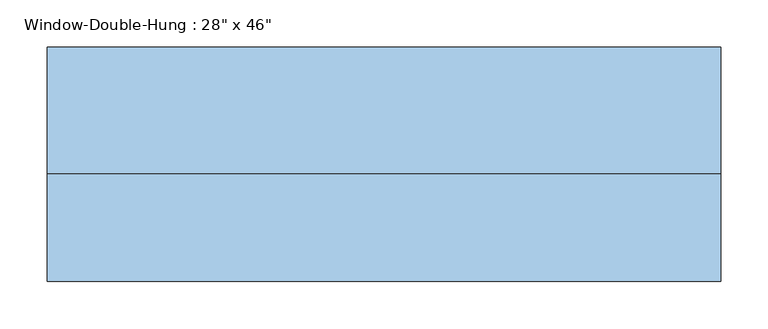
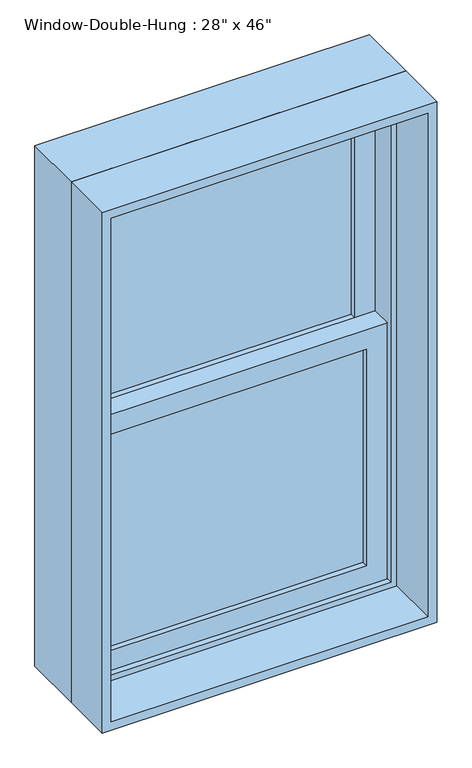
"""IFC4 building model written with IfcOpenShell, lengths in millimetres: window geometry."""

from ifc_helpers import new_model, si_unit, frame, origin, place, context, project, spatial, polyline, outline, extrude, source, transform, mapped, element, save


def window_fc4bf0c6(model_context):
    return source(origin(), model_context, "Body", "SweptSolid", [
        extrude(outline(polyline([(279.4, 44.45), (279.4, 38.1), (-279.4, 38.1), (-279.4, 44.45), (279.4, 44.45)])), frame((0.0, 0.0, 990.6), z_axis=(0.0, 0.0, 1.0), x_axis=(1.0, 0.0, 0.0)), (0.0, 0.0, 1.0), 485.775),
        extrude(outline(polyline([(-279.4, 31.75), (279.4, 31.75), (279.4, 25.4), (-279.4, 25.4), (-279.4, 31.75)])), frame((0.0, 0.0, 990.6), z_axis=(0.0, 0.0, 1.0), x_axis=(1.0, 0.0, 0.0)), (0.0, 0.0, 1.0), 485.775),
        extrude(outline(polyline([(279.4, 88.9), (279.4, 82.55), (-279.4, 82.55), (-279.4, 88.9), (279.4, 88.9)])), frame((0.0, 0.0, 1520.825), z_axis=(0.0, 0.0, 1.0), x_axis=(1.0, 0.0, 0.0)), (0.0, 0.0, 1.0), 485.775),
        extrude(outline(polyline([(-279.4, 76.2), (279.4, 76.2), (279.4, 69.85), (-279.4, 69.85), (-279.4, 76.2)])), frame((0.0, 0.0, 1520.825), z_axis=(0.0, 0.0, 1.0), x_axis=(1.0, 0.0, 0.0)), (0.0, 0.0, 1.0), 485.775),
        extrude(outline(polyline([(1520.825, -323.85), (946.15, -323.85), (946.15, 323.85), (1520.825, 323.85), (1520.825, -323.85)]), holes=[polyline([(1476.375, 279.4), (990.6, 279.4), (990.6, -279.4), (1476.375, -279.4), (1476.375, 279.4)])]), frame((0.0, 12.7, 0.0), z_axis=(0.0, 1.0, 0.0), x_axis=(0.0, 0.0, 1.0)), (0.0, 0.0, 1.0), 44.45),
        extrude(outline(polyline([(2051.05, -323.85), (1476.375, -323.85), (1476.375, 323.85), (2051.05, 323.85), (2051.05, -323.85)]), holes=[polyline([(2006.6, 279.4), (1520.825, 279.4), (1520.825, -279.4), (2006.6, -279.4), (2006.6, 279.4)])]), frame((0.0, 57.15, 0.0), z_axis=(0.0, 1.0, 0.0), x_axis=(0.0, 0.0, 1.0)), (0.0, 0.0, 1.0), 44.45),
        extrude(outline(polyline([(2082.8, -355.6), (914.4, -355.6), (914.4, 355.6), (2082.8, 355.6), (2082.8, -355.6)]), holes=[polyline([(2051.05, 323.85), (946.15, 323.85), (946.15, -323.85), (2051.05, -323.85), (2051.05, 323.85)])]), frame((0.0, 0.0, 0.0), z_axis=(0.0, 1.0, 0.0), x_axis=(0.0, 0.0, 1.0)), (0.0, 0.0, 1.0), 133.35),
        extrude(outline(polyline([(2082.8, 355.6), (2082.8, -355.6), (914.4, -355.6), (914.4, 355.6), (2082.8, 355.6)]), holes=[polyline([(2063.75, 336.55), (933.45, 336.55), (933.45, -336.55), (2063.75, -336.55), (2063.75, 336.55)])]), frame((0.0, -114.3, 0.0), z_axis=(0.0, 1.0, 0.0), x_axis=(0.0, 0.0, 1.0)), (0.0, 0.0, 1.0), 114.3),
    ])


if __name__ == "__main__":
    model = new_model("IFC4")
    model_context = context("Model", 3, world=origin())
    ifc_project = project(units=[si_unit("LENGTHUNIT", "METRE", prefix="MILLI")], contexts=[model_context])
    site = spatial("IfcSite", under=ifc_project)
    building = spatial("IfcBuilding", under=site)
    placement = place(None, origin())
    window_shape = window_fc4bf0c6(model_context)
    element("IfcWindow", 1, ObjectType="Window-Double-Hung : 28\" x 46\"", at=placement, inside=building, context=model_context, shape_type="MappedRepresentation", body=[
        mapped(window_shape, transform((0.0, 0.0, 0.0), x_axis=(1.0, 0.0, 0.0), y_axis=(0.0, 1.0, 0.0), z_axis=(0.0, 0.0, 1.0))),
    ])
    save(model, "model.ifc")

# Revit data of these elements
# Type "Window-Double-Hung : 28\" x 46\""
#   Type Mark = "12"
#   Fire Rating = "0.5h"
#   Construction Type Id = "DG-DR"
#   Assembly Code = "B2020100"
#   Analytic Construction = "Double glazing - domestic"
#   Wall Thickness [instance default] = 0' - 6"
#   Window Inset [instance default] = 0' - 0"
#   Visual Light Transmittance = 0.81
#   Thermal Resistance (R) = 1.8146 (h·ft²·°F)/BTU
#   Solar Heat Gain Coefficient = 0.76
#   Muntin Width = 1' - 10"
#   Muntin Height = 1' - 7 1/8"
#   Interior Wall Closure [instance default] = 0' - 1 1/2"
#   Rough Width = 2' - 4 1/2"
#   Rough Height = 3' - 10 1/2"
#   Frame Extension [instance default] = 0' - 1 1/4"
#   Exterior Wall Closure [instance default] = 0' - 0 1/2"
#   Extension Jamb [instance default] = 0' - 1 1/2"
#   Heat Transfer Coefficient (U) = 0.5511 BTU/(h·ft²·°F)
#   Height = 3' - 10"
#   Width = 2' - 4"
#   Define Thermal Properties by = 1
#   Top Muntin Visibility = yes
#   Indicator Visibility [instance default] = yes
#   Extension Jamb Visibility [instance default] = yes
#   Interior Trim Visibility [instance default] = yes
#   Exterior Trim Visibility [instance default] = yes
#   Define Thermal Properties by = 1
#   Bottom Muntin Visibility = yes
#   Muntin Pattern = Muntin Pattern_2x2 : Muntin Pattern_2x2
#   Interior Trim Material = Wood - Stained
#   Interior Trim = Trim-Window-Interior-Flat : Picture Frame
#   Exterior Trim Material = Clad - White
#   Exterior Trim = Trim-Window-Exterior-Flat : with Sill
#   Glass Panel Material = Glass
#   Exterior Frame Material = Clad - White
#   Interior Frame Material = Wood - Stained
#   Wall Closure = (empty or 0)
# Element 1 (IfcWindow, "Window-Double-Hung : 28\" x 46\"")
#   Wall Thickness = 0' - 9"
#   Extension Jamb = 0' - 4 1/2"
#   Materials on its faces: "Wood - Stained", "Glass", "Clad - White"
# Materials
#   "Wood - Stained": class "Wood", colour RGB 224 178 126, transparency 0, Cost = 0
#   "Clad - White": class "Wood", colour RGB 242 242 238, transparency 0, Cost = 0
#   "Glass": class "Glass", colour RGB 0 128 192, transparency 0.75, Description = "Soda Lime Glass", Cost = 0
